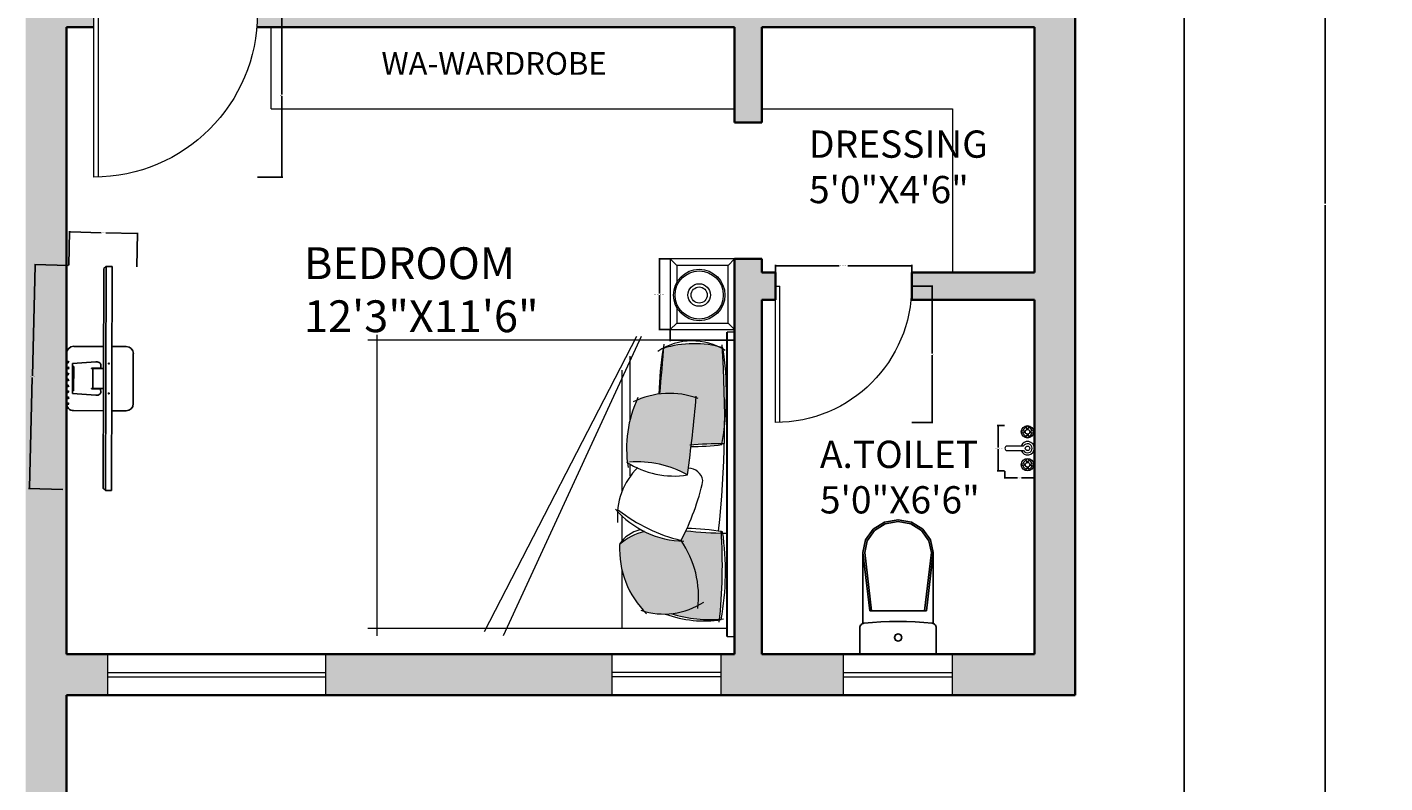
# Model space of a CAD drawing. Units: inches. Extents: x 3386 to 4477, y 1118 to 1824.
# Tile 4 of 7: x 3645 to 3944, y 1364 to 1530. Entities that reach past the tile are written whole.
import ezdxf

# ---------------------------------------------------------------- set-up
doc = ezdxf.new("R2010")
doc.units = ezdxf.units.IN
for name, color, linetype, lineweight in [('0.10', 252, 'Continuous', 9), ('0.15', 34, 'Continuous', 15), ('A-ANNO-DIMS', 2, 'Continuous', 18), ('A-ANNO-TEXT', 7, 'Continuous', 18), ('A-AREA-IDEN', 7, 'Continuous', 18), ('A-DOOR', 4, 'Continuous', 18), ('A-EQPM', 9, 'Continuous', 18), ('A-FLOR-CASE', 7, 'Continuous', 18), ('A-FURN', 8, 'Continuous', 18), ('A-GLAZ', 4, 'Continuous', 18), ('A-WALL', 7, 'Continuous', 35), ('C-PROP', 7, 'Continuous', 25), ('Сантехника', 7, 'Continuous', 18)]:
    doc.layers.add(name, color=color, linetype=linetype, lineweight=lineweight)
doc.layers.add('A-FURN-PATT', color=116, linetype='Continuous', lineweight=13, true_color=0x136734)
doc.layers.add('A-WALL-PATT', color=18, linetype='Continuous', lineweight=13, true_color=0x000000)
doc.layers.add('SANTEH', color=7, linetype='Continuous')
doc.layers.add('window', color=130, linetype='Continuous')
doc.styles.get("Standard").update_dxf_attribs({"font": 'arial.ttf'})
doc.dimstyles.get("Standard").update_dxf_attribs({"dimtxt": 0.18, "dimasz": 0.18, "dimexe": 0.18, "dimexo": 0.0625, "dimgap": 0.09, "dimtad": 0, "dimtih": 1, "dimtoh": 1, "dimdec": 4, "dimzin": 0, "dimdsep": 46, "dimtxsty": 'Standard', "dimcen": 0.09, "dimadec": 0, "dimazin": 0, "dimtfac": 1, "dimtdec": 4, "dimtofl": 0, "dimtmove": 0, "dimatfit": 3, "dimfxl": 1, "dimtolj": 1, "dimtzin": 0, "dimarcsym": 0})

# ---------------------------------------------------------------- blocks, each defined once
blk = doc.blocks.new('D1')
for p, q in [((0, 36), (0, 0)), ((1, 36), (1, 0)), ((0, 0), (1, 0))]:
    blk.add_line(p, q)
blk.add_arc((0, 0), 36, 0, 90)
blk = doc.blocks.new('D2')
for p, q in [((0, 30), (0, 0)), ((1, 30), (1, 0)), ((0, 0), (1, 0))]:
    blk.add_line(p, q)
blk.add_arc((0, 0), 30, 0, 90)
blk = doc.blocks.new('WC 2 Symb_109')
at = {"layer": 'SANTEH'}
for p, q in [((0, 0), (0, 380)), ((0, 380), (132.4, 380)), ((153.6, 364.9), (506.8, 364.9)), ((506.3, 364.9), (215.7, 330.9)), ((506.3, 356), (215.7, 322)), ((215.7, 190), (215.7, 330.9)), ((215.7, 190), (215.7, 49.1)), ((153.8, 15.1), (506.8, 15.1)), ((506.3, 24), (215.7, 58)), ((506.3, 15.1), (215.7, 49.1)), ((0, 0), (132.4, 0))]:
    blk.add_line(p, q, dxfattribs=at)
for points in [[(154.6, 360.1), (153.9, 364.1), (152.3, 367.9), (150.2, 371.3), (147.4, 374.3), (144.1, 376.7), (140.5, 378.5), (136.5, 379.6), (132.4, 380)], [(154.6, 19.7), (158.6, 62.1), (161.4, 104.7), (163.1, 147.3), (163.7, 189.9), (163.1, 232.5), (161.4, 275.1), (158.6, 317.7), (154.6, 360.1)], [(506.3, 24), (565.5, 36.6), (615.7, 72.6), (649.2, 126.5), (661, 190), (649.2, 253.5), (615.7, 307.4), (565.5, 343.4), (506.3, 356)], [(506.8, 15.1), (569.2, 28.4), (622.2, 66.3), (657.6, 123.1), (670, 190), (657.6, 256.9), (622.2, 313.7), (569.2, 351.6), (506.8, 364.9)], [(132.4, 0), (136.5, 0.4), (140.4, 1.5), (144.1, 3.2), (147.3, 5.6), (150.1, 8.6), (152.3, 12), (153.8, 15.7), (154.6, 19.7)]]:
    blk.add_lwpolyline(points, dxfattribs=at)
blk.add_lwpolyline([(83.6, 208.5), (70.4, 203.1), (64.9, 190), (70.4, 176.9), (83.6, 171.5), (96.8, 176.9), (102.2, 190), (96.8, 203.1)], close=True, dxfattribs=at)
blk = doc.blocks.new('Faucet - Bathroom top')
for p, q in [((-4.107, 0.125), (-4.375, 0.125)), ((-3.75, 0.4788), (-3.75, 0.75)), ((-3.5, 0.482), (-3.5, 0.75)), ((-3.1461, 0.125), (-2.875, 0.125)), ((3.143, 0.125), (2.875, 0.125)), ((3.5, 0.4788), (3.5, 0.75)), ((3.75, 0.482), (3.75, 0.75)), ((4.1039, 0.125), (4.375, 0.125)), ((-4.1039, -0.125), (-4.375, -0.125)), ((-3.75, -0.4821), (-3.75, -0.75)), ((-3.5, -0.4789), (-3.5, -0.75)), ((-3.143, -0.125), (-2.875, -0.125)), ((-0.5, -0.8639), (-0.5, -4.5)), ((0.5, -4.5), (0.5, -0.8631)), ((3.1461, -0.125), (2.875, -0.125)), ((3.5, -0.4821), (3.5, -0.75)), ((3.75, -0.4789), (3.75, -0.75)), ((4.107, -0.125), (4.375, -0.125))]:
    blk.add_line(p, q)
for centre, radius in [((-3.625, 0), 1.375), ((-4.625, 0), 0.2795), ((-3.625, 0), 0.5), ((-3.625, 1), 0.2795), ((-2.625, 0), 0.2795), ((0, 0), 0.5), ((3.625, 0), 1.375), ((2.625, 0), 0.2795), ((3.625, 0), 0.5), ((3.625, 1), 0.2795), ((4.625, 0), 0.2795), ((-3.625, -1), 0.2795), ((3.625, -1), 0.2795)]:
    blk.add_circle(centre, radius)
for centre, radius, start, end in [((-3.625, 0), 1, 105.2407, 164.2093), ((-3.625, 0), 1, 16.44125, 74.07887), ((0, 0), 1.5, 289.6514, 250.3603), ((0, 0), 1, 300.3431, 239.7554), ((3.625, 0), 1, 106.12, 164.0884), ((3.625, 0), 1, 16.23422, 73.90469), ((-3.625, 0), 1, 196.2342, 253.9047), ((-3.625, 0), 1, 286.12, 344.0884), ((3.625, 0), 1, 196.4413, 254.0789), ((3.625, 0), 1, 285.2407, 344.2093), ((0, -4.5), 0.5, 180, 0)]:
    blk.add_arc(centre, radius, start, end)
blk = doc.blocks.new('TV')
at = {"color": 0}
for p, q in [((3967.27, 1784.85), (3967.05, 1784.65)), ((3967.76, 1763.68), (3967.54, 1763.86))]:
    blk.add_line(p, q, dxfattribs=at)
at = {"layer": 'window'}
for p, q in [((3967.54, 1763.86), (3967.05, 1784.65)), ((3964.41, 1777.23), (3967.22, 1777.3)), ((3968.01, 1777.32), (3969.36, 1777.35)), ((3966.53, 1775.82), (3964.33, 1775.61)), ((3964.34, 1775.34), (3964.45, 1775.34)), ((3964.34, 1775.31), (3964.43, 1775.32)), ((3966.14, 1775.2), (3967.01, 1775.22)), ((3966.14, 1775.18), (3967.27, 1775.2)), ((3966.14, 1775.18), (3966.14, 1775.2)), ((3966.3, 1773.29), (3966.26, 1775.18)), ((3964.39, 1773.06), (3964.48, 1773.06)), ((3966.19, 1773.28), (3967.31, 1773.31)), ((3966.19, 1773.26), (3967.05, 1773.28)), ((3966.19, 1773.26), (3966.19, 1773.28)), ((3964.39, 1773.04), (3964.5, 1773.04)), ((3966.61, 1772.66), (3964.4, 1772.77)), ((3964.55, 1771.15), (3967.36, 1771.22)), ((3968.15, 1771.24), (3969.5, 1771.27))]:
    blk.add_line(p, q, dxfattribs=at)
for points in [[(3968.33, 1763.69), (3967.83, 1784.86), (3967.27, 1784.85), (3967.76, 1763.68), (3968.33, 1763.69)], [(3963.86, 1771.81), (3963.75, 1776.54)], [(3970.16, 1771.96), (3970.05, 1776.69)], [(3964.4, 1772.77), (3964.33, 1775.61)], [(3964.48, 1773.06), (3964.43, 1775.32)], [(3964.5, 1773.04), (3964.45, 1775.34)]]:
    blk.add_lwpolyline(points, dxfattribs=at)
for points in [[(3966.53, 1775.82, -0.263666), (3966.93, 1775.69), (3967, 1775.57), (3967.01, 1775.22)], [(3966.61, 1772.66, 0.263666), (3967, 1772.81), (3967.06, 1772.93), (3967.05, 1773.28)]]:
    blk.add_lwpolyline(points, format="xyb", dxfattribs=at)
for centre, radius in [((3963.91, 1775.73), 0.0679), ((3967.77, 1775.68), 0.0451), ((3963.93, 1775.17), 0.0679), ((3963.94, 1774.6), 0.0679), ((3963.95, 1774.04), 0.0679), ((3963.97, 1773.48), 0.0679), ((3963.98, 1772.92), 0.0679), ((3963.99, 1772.35), 0.0679), ((3964.01, 1771.79), 0.0679), ((3967.83, 1772.86), 0.0451)]:
    blk.add_circle(centre, radius, dxfattribs=at)
for centre, start, end in [((3964.42, 1776.56), 91.3414, 181.3414), ((3969.38, 1776.67), 1.3414, 91.3414), ((3964.53, 1771.83), 181.3414, 271.3414), ((3969.49, 1771.94), 271.3414, 1.3414)]:
    blk.add_arc(centre, 0.676, start, end, dxfattribs=at)
blk = doc.blocks.new('camita')
at = {"layer": '0.10'}
for p, q in [((-0.85, -0.045), (0.85, -0.045)), ((-0.805, -0.045), (-0.805, -2.0485)), ((0.805, -0.045), (0.805, -2.0485)), ((-0.8271, -0.521), (0.8464, -1.2932)), ((-0.8271, -0.5476), (0.8236, -1.3992)), ((-0.7161, -0.585), (-0.3554, -0.585)), ((-0.1136, -0.585), (-0.0485, -0.585)), ((-0.638, -0.63), (0.0434, -0.63)), ((0.1749, -0.63), (0.3179, -0.63)), ((0.4739, -0.63), (0.805, -0.63)), ((-0.8354, -2), (0.8464, -2))]:
    blk.add_line(p, q, dxfattribs=at)
blk.add_lwpolyline([(-0.85, -0.0405), (0.85, -0.0405), (0.85, 0), (-0.85, 0)], close=True, dxfattribs=at)
for centre, radius, start, end in [((-0.4574, -0.2364), 0.3443, 147.50996, 213.83359), ((-0.1997, -0.2266), 0.5864, 163.92635, 197.14087), ((-0.3639, -5.8457), 5.7909, 83.80731, 94.12107), ((-0.5104, -1.7232), 1.6781, 80.12554, 98.66187), ((2.3534, -0.0532), 2.5803, 180.10628, 184.38541), ((-1.5443, -0.2452), 1.3333, 359.93941, 7.55329), ((1.5815, -0.2893), 1.3353, 170.38021, 178.99138), ((-1.4396, -0.0609), 1.7117, 352.92911, 0.39592), ((0.4524, -3.0675), 2.9996, 83.90257, 93.67595), ((0.4863, -1.6286), 1.5781, 80.16015, 98.05996), ((0.0294, -0.1377), 0.7262, 342.58415, 6.00484), ((0.1326, -0.1696), 0.6307, 339.92303, 8.74334), ((-0.0543, -0.3633), 0.4542, 159.30257, 206.50263), ((-1.3301, -9.6748), 9.4985, 82.27078, 84.93989), ((-0.007, -0.258), 0.0828, 100.01798, 179.73597), ((-0.2931, -1.4378), 1.2903, 61.97485, 77.84351), ((0.6265, -0.7518), 0.5508, 82.96906, 124.67388), ((0.3203, -0.3944), 0.4043, 341.45245, 33.45121), ((0.4585, -0.5454), 0.5842, 151.04555, 184.14969), ((-0.5341, -0.3393), 0.4875, 327.26442, 9.0473), ((-0.1986, -0.2742), 0.5159, 310.73945, 359.05759), ((-0.5673, -0.0868), 0.9057, 321.69527, 346.46261), ((-1.8672, -14.986), 14.6323, 84.65974, 85.75157), ((-0.4598, 1.4861), 1.9092, 260.95299, 268.65169), ((0.4384, -0.4834), 0.1898, 193.68485, 236.70352), ((0.5707, -0.4317), 0.3145, 192.93877, 221.96363), ((0.3612, -0.133), 0.5096, 267.25889, 315.29965), ((-0.2002, 0.064), 0.6673, 244.78094, 279.06058), ((0.179, -0.272), 0.3828, 224.52836, 275.22287)]:
    blk.add_arc(centre, radius, start, end, dxfattribs=at)
blk = doc.blocks.new('VELADOR')
at = {"layer": '0.15'}
for p, q in [((-0.2475, 0), (-0.2025, -0.045)), ((0.2475, 0), (0.2025, -0.045)), ((-0.2025, -0.405), (-0.2475, -0.45)), ((0.2475, -0.45), (0.2025, -0.405))]:
    blk.add_line(p, q, dxfattribs=at)
blk.add_lwpolyline([(-0.2475, 0), (-0.2475, -0.45), (0.2475, -0.45), (0.2475, 0)], close=True, dxfattribs=at)
blk.add_lwpolyline([(0.0921, -0.405), (0.2025, -0.405), (0.2025, -0.045), (-0.2025, -0.045), (-0.2025, -0.405), (-0.0818, -0.405)], dxfattribs=at)
for radius in [0.18, 0.1688, 0.0788, 0.0563]:
    blk.add_circle((0.0052, -0.2474), radius, dxfattribs=at)
blk = doc.blocks.new('WIN-24IN')
for p, q in [((0, 0), (0, 9)), ((24, 0), (24, 9)), ((0, 5), (24, 5)), ((0, 4), (24, 4))]:
    blk.add_line(p, q)
blk = doc.blocks.new('WIN-48IN')
for p, q in [((0, 48), (9, 48)), ((4, 0), (4, 48)), ((5, 0), (5, 48)), ((0, 0), (9, 0))]:
    blk.add_line(p, q)
blk = doc.blocks.new('WARDROBE-102IN')
for q in [(0, 18), (102, 0)]:
    blk.add_line((0, 0), q)
blk = doc.blocks.new('DRESSING-UNIT-42X36')
for p, q in [((0, 36), (42, 36)), ((42, 36), (42, 0))]:
    blk.add_line(p, q)
blk = doc.blocks.new('*D66')
at = {"layer": 'A-ANNO-DIMS', "color": 0, "lineweight": -2, "transparency": 16777216}
for p, q in [((3695.72, 1532.87), (3701.24, 1532.87)), ((3701.06, 1532.69), (3701.06, 1515.05)), ((3701.06, 1497.05), (3701.06, 1514.69)), ((3695.72, 1496.87), (3701.24, 1496.87))]:
    blk.add_line(p, q, dxfattribs=at)
at = {"layer": 'A-ANNO-DIMS', "color": 0, "transparency": 16777216}
for points in [[(3701.03, 1532.69), (3701.09, 1532.69), (3701.06, 1532.87)], [(3701.03, 1497.05), (3701.09, 1497.05), (3701.06, 1496.87)]]:
    blk.add_solid(points, dxfattribs=at)
at = {"layer": 'Defpoints', "color": 0, "transparency": 16777216}
for p in [(3695.66, 1532.87), (3695.66, 1496.87), (3701.06, 1496.87)]:
    blk.add_point(p, dxfattribs=at)
at = {"layer": 'A-ANNO-DIMS', "color": 0, "transparency": 16777216, "insert": (3701.06, 1514.87), "char_height": 0.18, "attachment_point": 5}
blk.add_mtext('\\A1;36 TYP.', dxfattribs=at)
blk = doc.blocks.new('*D67')
at = {"layer": 'A-ANNO-DIMS', "color": 0, "lineweight": -2, "transparency": 16777216}
for p, q in [((3809.66, 1472.93), (3809.66, 1477.55)), ((3809.84, 1477.37), (3823.72, 1477.37)), ((3839.48, 1477.37), (3825.59, 1477.37)), ((3839.66, 1472.93), (3839.66, 1477.55))]:
    blk.add_line(p, q, dxfattribs=at)
at = {"layer": 'A-ANNO-DIMS', "color": 0, "transparency": 16777216}
for points in [[(3809.84, 1477.4), (3809.84, 1477.34), (3809.66, 1477.37)], [(3839.48, 1477.4), (3839.48, 1477.34), (3839.66, 1477.37)]]:
    blk.add_solid(points, dxfattribs=at)
at = {"layer": 'Defpoints', "color": 0, "transparency": 16777216}
for p in [(3839.66, 1477.37), (3809.66, 1472.87), (3839.66, 1472.87)]:
    blk.add_point(p, dxfattribs=at)
at = {"layer": 'A-ANNO-DIMS', "color": 0, "transparency": 16777216, "insert": (3824.66, 1477.37), "char_height": 0.18, "attachment_point": 5}
blk.add_mtext('\\A1;DOOR 30 TYP.', dxfattribs=at)
blk = doc.blocks.new('*D68')
at = {"layer": 'A-ANNO-DIMS', "color": 0, "lineweight": -2, "transparency": 16777216}
for p, q in [((3839.72, 1472.87), (3844.34, 1472.87)), ((3844.16, 1472.69), (3844.16, 1458.05)), ((3844.16, 1443.05), (3844.16, 1457.69)), ((3839.72, 1442.87), (3844.34, 1442.87))]:
    blk.add_line(p, q, dxfattribs=at)
at = {"layer": 'A-ANNO-DIMS', "color": 0, "transparency": 16777216}
for points in [[(3844.13, 1472.69), (3844.19, 1472.69), (3844.16, 1472.87)], [(3844.13, 1443.05), (3844.19, 1443.05), (3844.16, 1442.87)]]:
    blk.add_solid(points, dxfattribs=at)
at = {"layer": 'Defpoints', "color": 0, "transparency": 16777216}
for p in [(3839.66, 1472.87), (3839.66, 1442.87), (3844.16, 1442.87)]:
    blk.add_point(p, dxfattribs=at)
at = {"layer": 'A-ANNO-DIMS', "color": 0, "transparency": 16777216, "insert": (3844.16, 1457.87), "char_height": 0.18, "attachment_point": 5}
blk.add_mtext('\\A1;30 TYP.', dxfattribs=at)
blk = doc.blocks.new('*D75')
at = {"layer": 'A-ANNO-DIMS', "color": 0, "lineweight": -2, "transparency": 16777216}
for p, q in [((3786.46, 1478.87), (3784.01, 1478.87)), ((3784.19, 1478.69), (3784.19, 1471.28)), ((3784.19, 1463.5), (3784.19, 1470.91)), ((3786.46, 1463.32), (3784.01, 1463.32))]:
    blk.add_line(p, q, dxfattribs=at)
at = {"layer": 'A-ANNO-DIMS', "color": 0, "transparency": 16777216}
for points in [[(3784.16, 1478.69), (3784.22, 1478.69), (3784.19, 1478.87)], [(3784.16, 1463.5), (3784.22, 1463.5), (3784.19, 1463.32)]]:
    blk.add_solid(points, dxfattribs=at)
at = {"layer": 'Defpoints', "color": 0, "transparency": 16777216}
for p in [(3786.52, 1478.87), (3784.19, 1463.32), (3786.52, 1463.32)]:
    blk.add_point(p, dxfattribs=at)
at = {"layer": 'A-ANNO-DIMS', "color": 0, "transparency": 16777216, "insert": (3784.19, 1471.09), "char_height": 0.18, "attachment_point": 5}
blk.add_mtext('\\A1;NIGHTSTAND 16 TYP.', dxfattribs=at)
blk = doc.blocks.new('*D76')
at = {"layer": 'A-ANNO-DIMS', "color": 0, "lineweight": -2, "transparency": 16777216}
for p, q in [((3786.52, 1463.25), (3786.52, 1460.8)), ((3800.66, 1463.25), (3800.66, 1460.8)), ((3786.7, 1460.98), (3793.07, 1460.98)), ((3800.48, 1460.98), (3794.11, 1460.98))]:
    blk.add_line(p, q, dxfattribs=at)
at = {"layer": 'A-ANNO-DIMS', "color": 0, "transparency": 16777216}
for points in [[(3786.7, 1461.01), (3786.7, 1460.95), (3786.52, 1460.98)], [(3800.48, 1461.01), (3800.48, 1460.95), (3800.66, 1460.98)]]:
    blk.add_solid(points, dxfattribs=at)
at = {"layer": 'Defpoints', "color": 0, "transparency": 16777216}
for p in [(3786.52, 1463.32), (3800.66, 1463.32), (3800.66, 1460.98)]:
    blk.add_point(p, dxfattribs=at)
at = {"layer": 'A-ANNO-DIMS', "color": 0, "transparency": 16777216, "insert": (3793.59, 1460.98), "char_height": 0.18, "attachment_point": 5}
blk.add_mtext('\\A1;14 TYP.', dxfattribs=at)
blk = doc.blocks.new('*D79')
at = {"layer": 'A-ANNO-DIMS', "color": 0, "lineweight": -2, "transparency": 16777216}
for p, q in [((3860.09, 1442.2), (3858.48, 1442.2)), ((3858.66, 1442.02), (3858.66, 1437.38)), ((3858.66, 1432.38), (3858.66, 1437.02)), ((3860.09, 1432.2), (3858.48, 1432.2))]:
    blk.add_line(p, q, dxfattribs=at)
at = {"layer": 'A-ANNO-DIMS', "color": 0, "transparency": 16777216}
for points in [[(3858.63, 1442.02), (3858.69, 1442.02), (3858.66, 1442.2)], [(3858.63, 1432.38), (3858.69, 1432.38), (3858.66, 1432.2)]]:
    blk.add_solid(points, dxfattribs=at)
at = {"layer": 'Defpoints', "color": 0, "transparency": 16777216}
for p in [(3860.16, 1442.2), (3858.66, 1432.2), (3860.16, 1432.2)]:
    blk.add_point(p, dxfattribs=at)
at = {"layer": 'A-ANNO-DIMS', "color": 0, "transparency": 16777216, "insert": (3858.66, 1437.2), "char_height": 0.18, "attachment_point": 5}
blk.add_mtext('\\A1;BATH TAP 10 TYP.', dxfattribs=at)
blk = doc.blocks.new('*D80')
at = {"layer": 'A-ANNO-DIMS', "color": 0, "lineweight": -2, "transparency": 16777216}
for p, q in [((3860.16, 1432.14), (3860.16, 1430.52)), ((3866.66, 1432.14), (3866.66, 1430.52)), ((3860.34, 1430.7), (3862.95, 1430.7)), ((3866.48, 1430.7), (3863.86, 1430.7))]:
    blk.add_line(p, q, dxfattribs=at)
at = {"layer": 'A-ANNO-DIMS', "color": 0, "transparency": 16777216}
for points in [[(3860.34, 1430.73), (3860.34, 1430.67), (3860.16, 1430.7)], [(3866.48, 1430.73), (3866.48, 1430.67), (3866.66, 1430.7)]]:
    blk.add_solid(points, dxfattribs=at)
at = {"layer": 'Defpoints', "color": 0, "transparency": 16777216}
for p in [(3860.16, 1432.2), (3866.66, 1432.2), (3866.66, 1430.7)]:
    blk.add_point(p, dxfattribs=at)
at = {"layer": 'A-ANNO-DIMS', "color": 0, "transparency": 16777216, "insert": (3863.41, 1430.7), "char_height": 0.18, "attachment_point": 5}
blk.add_mtext('\\A1;7 TYP.', dxfattribs=at)
blk = doc.blocks.new('*D81')
at = {"layer": 'A-ANNO-DIMS', "color": 0, "lineweight": -2, "transparency": 16777216}
for p, q in [((3646.75, 1477.43), (3646.13, 1453.15)), ((3654.09, 1477.43), (3646.58, 1477.62)), ((3645.51, 1428.51), (3646.12, 1452.79)), ((3652.83, 1428.14), (3645.32, 1428.33))]:
    blk.add_line(p, q, dxfattribs=at)
at = {"layer": 'A-ANNO-DIMS', "color": 0, "transparency": 16777216}
for points in [[(3646.72, 1477.44), (3646.78, 1477.43), (3646.76, 1477.61)], [(3645.48, 1428.51), (3645.54, 1428.51), (3645.5, 1428.33)]]:
    blk.add_solid(points, dxfattribs=at)
at = {"layer": 'Defpoints', "color": 0, "transparency": 16777216}
for p in [(3646.76, 1477.61), (3654.15, 1477.43), (3652.9, 1428.14)]:
    blk.add_point(p, dxfattribs=at)
at = {"layer": 'A-ANNO-DIMS', "color": 0, "transparency": 16777216, "insert": (3646.13, 1452.97), "char_height": 0.18, "attachment_point": 5}
blk.add_mtext('\\A1;TV 49 TYP.', dxfattribs=at)
blk = doc.blocks.new('*D82')
at = {"layer": 'A-ANNO-DIMS', "color": 0, "lineweight": -2, "transparency": 16777216}
for p, q in [((3654.15, 1477.49), (3654.34, 1485)), ((3654.52, 1484.82), (3661.29, 1484.64)), ((3669.11, 1484.44), (3662.33, 1484.62)), ((3669.1, 1477.11), (3669.29, 1484.62))]:
    blk.add_line(p, q, dxfattribs=at)
at = {"layer": 'A-ANNO-DIMS', "color": 0, "transparency": 16777216}
for points in [[(3654.52, 1484.85), (3654.52, 1484.79), (3654.34, 1484.82)], [(3669.11, 1484.47), (3669.11, 1484.41), (3669.29, 1484.44)]]:
    blk.add_solid(points, dxfattribs=at)
at = {"layer": 'Defpoints', "color": 0, "transparency": 16777216}
for p in [(3669.29, 1484.44), (3654.15, 1477.43), (3669.1, 1477.05)]:
    blk.add_point(p, dxfattribs=at)
at = {"layer": 'A-ANNO-DIMS', "color": 0, "transparency": 16777216, "insert": (3661.81, 1484.63), "char_height": 0.18, "attachment_point": 5}
blk.add_mtext('\\A1;15 TYP.', dxfattribs=at)
blk = doc.blocks.new('*D106')
at = {"layer": 'A-ANNO-DIMS', "color": 0, "lineweight": -2, "transparency": 16777216}
for p, q in [((3963.65, 1790.87), (3930.48, 1790.87)), ((3930.66, 1790.69), (3930.66, 1491.05)), ((3930.66, 1191.05), (3930.66, 1490.69)), ((3963.65, 1190.87), (3930.48, 1190.87))]:
    blk.add_line(p, q, dxfattribs=at)
at = {"layer": 'A-ANNO-DIMS', "color": 0, "transparency": 16777216}
for points in [[(3930.63, 1790.69), (3930.69, 1790.69), (3930.66, 1790.87)], [(3930.63, 1191.05), (3930.69, 1191.05), (3930.66, 1190.87)]]:
    blk.add_solid(points, dxfattribs=at)
at = {"layer": 'Defpoints', "color": 0, "transparency": 16777216}
for p in [(3930.66, 1790.87), (3963.71, 1790.87), (3963.71, 1190.87)]:
    blk.add_point(p, dxfattribs=at)
at = {"layer": 'A-ANNO-DIMS', "color": 0, "transparency": 16777216, "insert": (3930.66, 1490.87), "char_height": 0.18, "attachment_point": 5}
blk.add_mtext('\\A1;600', dxfattribs=at)

msp = doc.modelspace()

# ---------------------------------------------------------------- hatches: boundary and pattern name
at = {"layer": 'A-FURN-PATT'}
h = msp.add_hatch(color=256, dxfattribs=at)
h.dxf.hatch_style = 1
h.paths.add_polyline_path([(3784.23, 1449.16, -0.113891), (3792.22, 1448.29, -0.006967), (3791.15, 1437.93, -0.016701), (3797.93, 1438.19, 0.015442), (3798.5, 1442.23, 0.01851), (3797.97, 1459.1, 0.020657), (3796.97, 1459.61, 0.131047), (3785.08, 1459.23, -0.004387)])
h.paths.add_polyline_path([(3789.96, 1419.06, -0.011742), (3788.89, 1416.93, -0.175864), (3792.65, 1402.62, -0.098488), (3786.71, 1400.81, 0.094792), (3797.39, 1399.59, 0.040212), (3797.77, 1418.55, -0.029051)])
h = msp.add_hatch(color=256, dxfattribs=at)
h.dxf.hatch_style = 1
h.paths.add_polyline_path([(3779.14, 1447.82, -0.189536), (3792.22, 1448.34, -0.011408), (3790.31, 1431.38, 0.150361), (3777.07, 1434.16, -0.133776)])
h.paths.add_polyline_path([(3792.64, 1402.67, -0.194952), (3780.75, 1401.38, -0.202559), (3775.37, 1416.05, -0.127326), (3780.88, 1418.91, 0.104045), (3788.98, 1416.84, -0.173835)])
at = {"layer": 'A-WALL-PATT'}
h = msp.add_hatch(color=256, dxfattribs=at)
h.dxf.hatch_style = 1
h.paths.add_polyline_path([(3443.66, 1221.87), (3452.66, 1221.87), (3452.66, 1301.87), (3458.66, 1301.87), (3458.66, 1310.87), (3452.66, 1310.87), (3452.66, 1328.87), (3443.66, 1328.87)])
h.paths.add_polyline_path([(3506.66, 1310.87), (3506.66, 1306.37), (3506.66, 1301.87), (3530.66, 1301.87), (3530.66, 1310.87)])
h.paths.add_polyline_path([(3653.66, 1301.87), (3653.66, 1382.87), (3662.66, 1382.87), (3662.66, 1391.87), (3653.66, 1391.87), (3653.66, 1529.87), (3659.66, 1529.87), (3659.66, 1535.87), (3644.66, 1535.87), (3644.66, 1310.87), (3602.66, 1310.87), (3602.66, 1301.87)])
h.paths.add_polyline_path([(3452.66, 1406.87), (3443.66, 1406.87), (3443.66, 1376.87), (3452.66, 1376.87), (3452.66, 1388.44)])
h.paths.add_polyline_path([(3452.66, 1478.87), (3452.66, 1502.87), (3478.74, 1502.87), (3482.66, 1502.87), (3482.66, 1504.87), (3482.66, 1517.87), (3473.66, 1517.87), (3473.66, 1511.87), (3443.66, 1511.87), (3443.66, 1478.87)])
h.paths.add_polyline_path([(3773.66, 1391.87), (3710.66, 1391.87), (3710.66, 1382.87), (3773.66, 1382.87)], flags=17)
h.paths.add_polyline_path([(3824.66, 1391.87), (3806.66, 1391.87), (3806.66, 1469.87), (3809.66, 1469.87), (3809.66, 1472.87), (3809.66, 1475.87), (3806.66, 1475.87), (3806.66, 1478.87), (3800.66, 1478.87), (3800.66, 1463.32), (3800.66, 1391.87), (3797.66, 1391.87), (3797.66, 1382.87), (3824.66, 1382.87)], flags=17)
h.paths.add_polyline_path([(3866.66, 1469.87), (3866.66, 1391.87), (3848.66, 1391.87), (3848.66, 1382.87), (3875.66, 1382.87), (3875.66, 1547.87), (3866.66, 1547.87), (3866.66, 1535.87), (3695.66, 1535.87), (3695.66, 1529.87), (3800.66, 1529.87), (3800.66, 1508.87), (3806.66, 1508.87), (3806.66, 1529.87), (3866.66, 1529.87), (3866.66, 1475.87), (3839.66, 1475.87), (3839.66, 1469.87)])
h.paths.add_polyline_path([(3875.66, 1673.87), (3866.66, 1673.87), (3866.66, 1663.37), (3866.66, 1647.44), (3866.66, 1613.87), (3761.66, 1613.87), (3761.66, 1607.87), (3866.66, 1607.87), (3866.66, 1595.87), (3875.66, 1595.87)])
h.paths.add_polyline_path([(3473.66, 1607.87), (3473.66, 1601.87), (3482.66, 1601.87), (3482.66, 1616.87), (3452.66, 1616.87), (3452.66, 1640.87), (3443.66, 1640.87), (3443.66, 1607.87)])
h.paths.add_polyline_path([(3491.66, 1736.87), (3491.66, 1745.87), (3478.95, 1745.87), (3443.66, 1745.87), (3443.66, 1688.87), (3452.66, 1688.87), (3452.66, 1736.87)])
h.paths.add_polyline_path([(3551.66, 1745.87), (3539.66, 1745.87), (3539.66, 1736.87), (3551.66, 1736.87)])
h.paths.add_polyline_path([(3587.66, 1745.87), (3581.66, 1745.87), (3581.66, 1741.37), (3581.66, 1736.87), (3587.66, 1736.87), (3587.66, 1712.87), (3596.66, 1712.87), (3596.66, 1757.87), (3644.66, 1757.87), (3644.66, 1679.87), (3596.66, 1679.87), (3596.66, 1682.87), (3592.16, 1682.87), (3587.66, 1682.87), (3587.66, 1607.87), (3602.66, 1607.87), (3602.66, 1613.87), (3596.66, 1613.87), (3596.66, 1673.87), (3644.66, 1673.87), (3644.66, 1613.87), (3638.66, 1613.87), (3638.66, 1610.87), (3638.66, 1607.87), (3725.66, 1607.87), (3725.66, 1613.87), (3722.66, 1613.87), (3722.66, 1634.87), (3716.66, 1634.87), (3716.66, 1613.87), (3650.66, 1613.87), (3650.66, 1673.87), (3683.66, 1673.87), (3683.66, 1679.87), (3650.66, 1679.87), (3650.66, 1757.87), (3671.66, 1757.87), (3671.66, 1766.87), (3587.66, 1766.87)])
h.paths.add_polyline_path([(3716.66, 1757.87), (3716.66, 1679.87), (3713.66, 1679.87), (3713.66, 1673.87), (3716.66, 1673.87), (3716.66, 1664.87), (3722.66, 1664.87), (3722.66, 1757.87), (3728.66, 1757.87), (3728.66, 1766.87), (3695.66, 1766.87), (3695.66, 1757.87)])
h.paths.add_polyline_path([(3806.66, 1757.87), (3806.66, 1766.87), (3776.66, 1766.87), (3776.66, 1757.87)])
h.paths.add_polyline_path([(3875.66, 1766.87), (3854.66, 1766.87), (3854.66, 1757.87), (3866.66, 1757.87), (3866.66, 1733.87), (3875.66, 1733.87)])

# ---------------------------------------------------------------- linework, layer by layer
at = {"layer": 'A-WALL'}
for p, q in [((3875.66, 1766.87), (3875.66, 1382.87)), ((3653.66, 1529.87), (3659.66, 1529.87)), ((3653.66, 1391.87), (3653.66, 1529.87)), ((3695.66, 1529.87), (3800.66, 1529.87)), ((3800.66, 1529.87), (3800.66, 1508.87)), ((3806.66, 1529.87), (3806.66, 1508.87)), ((3806.66, 1529.87), (3866.66, 1529.87)), ((3866.66, 1529.87), (3866.66, 1475.87)), ((3800.66, 1508.87), (3806.66, 1508.87)), ((3800.66, 1478.87), (3806.66, 1478.87)), ((3800.66, 1478.87), (3800.66, 1391.87)), ((3806.66, 1478.87), (3806.66, 1475.87)), ((3806.66, 1475.87), (3809.66, 1475.87)), ((3809.66, 1475.87), (3809.66, 1469.87)), ((3839.66, 1475.87), (3839.66, 1469.87)), ((3839.66, 1475.87), (3866.66, 1475.87)), ((3806.66, 1469.87), (3809.66, 1469.87)), ((3806.66, 1469.87), (3806.66, 1391.87)), ((3839.66, 1469.87), (3866.66, 1469.87)), ((3866.66, 1469.87), (3866.66, 1391.87)), ((3653.66, 1391.87), (3800.66, 1391.87)), ((3806.66, 1391.87), (3866.66, 1391.87)), ((3653.66, 1301.87), (3653.66, 1382.87)), ((3653.66, 1382.87), (3875.66, 1382.87))]:
    msp.add_line(p, q, dxfattribs=at)
at = {"layer": 'C-PROP'}
msp.add_lwpolyline([(3419.66, 1790.87), (3899.66, 1790.87), (3899.66, 1190.87), (3419.66, 1190.87)], close=True, dxfattribs=at)

# ---------------------------------------------------------------- block references
at = {"layer": 'A-DOOR', "xscale": -1, "rotation": 180}
for name, p in [('D1', (3659.66, 1532.87)), ('D2', (3809.66, 1472.87))]:
    msp.add_blockref(name, p, dxfattribs=at)
at = {"layer": 'A-EQPM', "xscale": 2.327319231123021, "yscale": 2.327319231123021, "zscale": 2.327319231123021, "rotation": 358.5430845181613}
msp.add_blockref('TV', (-5673.37, -2440.63), dxfattribs=at)
at = {"layer": 'A-FLOR-CASE'}
for name, p in [('WARDROBE-102IN', (3698.66, 1511.87)), ('DRESSING-UNIT-42X36', (3806.66, 1475.87))]:
    msp.add_blockref(name, p, dxfattribs=at)
at = {"layer": 'A-FURN', "rotation": 270}
for name, p, xscale, yscale, zscale in [('VELADOR', (3800.66, 1471.09), 31.41542173157097, 31.41542173157097, 31.41542173157097), ('camita', (3800.66, 1429.26), 39.375, 39.375, 39.375)]:
    msp.add_blockref(name, p, dxfattribs=dict(at, xscale=xscale, yscale=yscale, zscale=zscale))
at = {"layer": 'A-GLAZ'}
for name, p, rotation in [('WIN-48IN', (3662.66, 1391.87), 269.9999999999994), ('WIN-24IN', (3797.66, 1391.87), 180)]:
    msp.add_blockref(name, p, dxfattribs=dict(at, rotation=rotation))
msp.add_blockref('WIN-24IN', (3824.66, 1382.87), dxfattribs=at)
at = {"layer": 'Сантехника', "rotation": 270}
msp.add_blockref('Faucet - Bathroom top', (3865.16, 1437.2), dxfattribs=at)
at = {"layer": 'Сантехника', "xscale": -0.0441898926459964, "yscale": 0.0441898926459964, "zscale": 0.0441898926459964, "rotation": 270.0000000000001}
msp.add_blockref('WC 2 Symb_109', (3828.26, 1391.87), dxfattribs=at)

# ---------------------------------------------------------------- texts
at = {"layer": 'A-ANNO-TEXT', "insert": (3722.96, 1524.38), "char_height": 5, "attachment_point": 1}
msp.add_mtext_dynamic_manual_height_columns('{\\fTimes New Roman|b0|i0|c0|p18;WA-WARDROBE}', width=79.5604, gutter_width=12.5, heights=[0], dxfattribs=at)
at = {"layer": 'A-AREA-IDEN', "attachment_point": 1}
for s, insert, char_height in [('{\\fTimes New Roman|b0|i0|c0|p18;DRESSING\\P5\'0"X4\'6"}', (3817.05, 1507.13), 6), ('{\\fTimes New Roman|b0|i0|c0|p18;BEDROOM\\P12\'3"X11\'6"}', (3705.91, 1481.42), 7), ('{\\fTimes New Roman|b0|i0|c0|p18;A.TOILET\\P5\'0"X6\'6"}', (3819.46, 1438.86), 6)]:
    msp.add_mtext_dynamic_manual_height_columns(s, width=79.5604, gutter_width=12.5, heights=[0], dxfattribs=dict(at, insert=insert, char_height=char_height))

# ---------------------------------------------------------------- dimensions: what is measured, and where the dimension line sits
at = {"layer": 'A-ANNO-DIMS'}
dim = msp.add_linear_dim(base=(3930.66, 1790.87), p1=(3963.71, 1190.87), p2=(3963.71, 1790.87), angle=90, dimstyle='Standard', override={"dimdec": 0, "dimlfac": 1, "dimrnd": 0, "dimzin": 0, "dimdsep": 46, "dimlunit": 2}, dxfattribs=at)
dim.commit()
dim.dimension.update_dxf_attribs({"geometry": '*D106', "text_midpoint": (3930.66, 1490.87)})
for base, p1, p2, angle, text, picture, middle in [((3701.06, 1496.87), (3695.66, 1532.87), (3695.66, 1496.87), 270, '<> TYP.', '*D66', (3701.06, 1514.87)), ((3669.29, 1484.44), (3654.15, 1477.43), (3669.1, 1477.05), 358.5431, '<> TYP.', '*D82', (3661.81, 1484.63)), ((3646.76, 1477.61), (3652.9, 1428.14), (3654.15, 1477.43), 88.5431, 'TV <> TYP.', '*D81', (3646.13, 1452.97)), ((3784.19, 1463.32), (3786.52, 1478.87), (3786.52, 1463.32), 270, 'NIGHTSTAND <> TYP.', '*D75', (3784.19, 1471.09)), ((3844.16, 1442.87), (3839.66, 1472.87), (3839.66, 1442.87), 270, '<> TYP.', '*D68', (3844.16, 1457.87)), ((3858.66, 1432.2), (3860.16, 1442.2), (3860.16, 1432.2), 270, 'BATH TAP <> TYP.', '*D79', (3858.66, 1437.2))]:
    dim = msp.add_linear_dim(base=base, p1=p1, p2=p2, angle=angle, text=text, dimstyle='Standard', override={"dimdec": 0, "dimlfac": 1, "dimrnd": 0, "dimzin": 0, "dimdsep": 46, "dimlunit": 2}, dxfattribs=at)
    dim.commit()
    dim.dimension.update_dxf_attribs({"geometry": picture, "text_midpoint": middle})
for base, p1, p2, text, picture, middle in [((3839.66, 1477.37), (3809.66, 1472.87), (3839.66, 1472.87), 'DOOR <> TYP.', '*D67', (3824.66, 1477.37)), ((3800.66, 1460.98), (3786.52, 1463.32), (3800.66, 1463.32), '<> TYP.', '*D76', (3793.59, 1460.98)), ((3866.6554, 1430.7015), (3860.1553, 1432.2015), (3866.6554, 1432.2015), '<> TYP.', '*D80', (3863.4053, 1430.7015))]:
    dim = msp.add_linear_dim(base=base, p1=p1, p2=p2, text=text, dimstyle='Standard', override={"dimdec": 0, "dimlfac": 1, "dimrnd": 0, "dimzin": 0, "dimdsep": 46, "dimlunit": 2}, dxfattribs=at)
    dim.commit()
    dim.dimension.update_dxf_attribs({"geometry": picture, "text_midpoint": middle})

doc.saveas('drawing.dxf')
